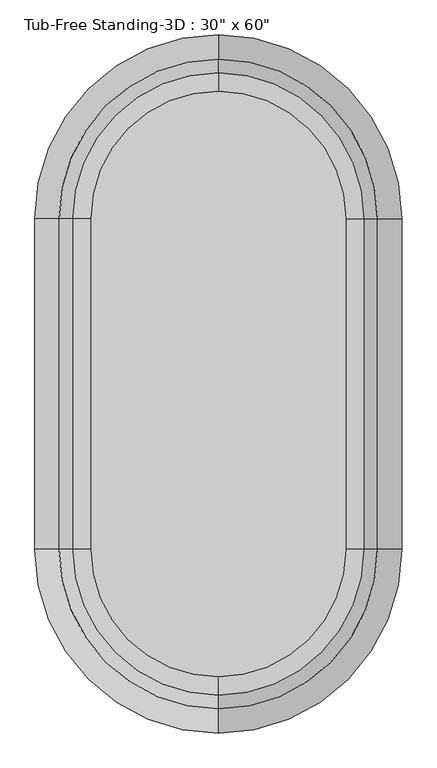
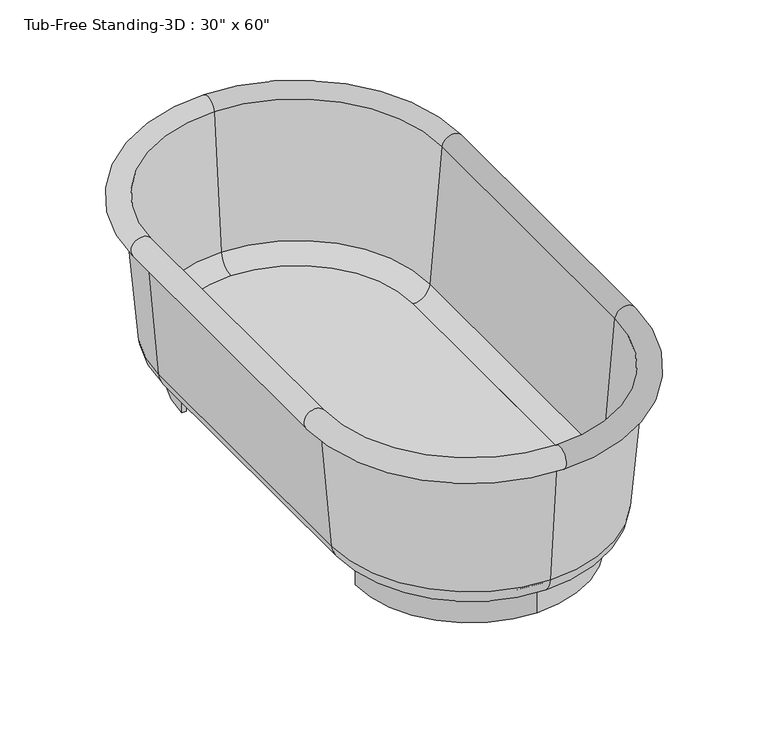
"""IFC4 building model written with IfcOpenShell, lengths in millimetres: flow terminal geometry."""

from ifc_helpers import new_model, si_unit, point, frame, frame_2d, origin, origin_with_axes, place, context, project, spatial, polyline, circle_curve, ellipse_curve, trimmed, segment, composite_curve, outline, extrude, source, transform, mapped, element, save
from ifc_brep_helpers import plane_surface, cylinder_surface, revolved_surface, advanced_brep


def flow_terminal_db991eef(model_context):
    return source(origin(), model_context, "Body", "SolidModel", [
        extrude(outline(composite_curve([segment(trimmed(circle_curve(frame_2d((0.0, 342.9)), 254.0), [point((0.0, 596.9))], [point((-254.0, 342.9))], True, "CARTESIAN"), True, "CONTINUOUS"), segment(polyline([(-254.0, 342.9), (-264.2824236, 342.9)]), True, "CONTINUOUS"), segment(trimmed(circle_curve(frame_2d((0.0, 342.9)), 264.2824236), [point((-264.2824236, 342.9))], [point((0.0, 607.1824236))], False, "CARTESIAN"), True, "CONTINUOUS"), segment(trimmed(circle_curve(frame_2d((0.0, 342.9)), 264.2824236), [point((0.0, 607.1824236))], [point((264.2824236, 342.9))], False, "CARTESIAN"), True, "CONTINUOUS"), segment(polyline([(264.2824236, 342.9), (254.0, 342.9)]), True, "CONTINUOUS"), segment(trimmed(circle_curve(frame_2d((0.0, 342.9)), 254.0), [point((254.0, 342.9))], [point((0.0, 596.9))], True, "CARTESIAN"), True, "CONTINUOUS")], self_intersect=False)), origin_with_axes(), (0.0, 0.0, 1.0), 63.5),
        extrude(outline(composite_curve([segment(trimmed(circle_curve(frame_2d((0.0, -342.9)), 264.2824236), [point((0.0, -607.1824236))], [point((-264.2824236, -342.9))], False, "CARTESIAN"), True, "CONTINUOUS"), segment(polyline([(-264.2824236, -342.9), (-254.0, -342.9)]), True, "CONTINUOUS"), segment(trimmed(circle_curve(frame_2d((0.0, -342.9)), 254.0), [point((-254.0, -342.9))], [point((0.0, -596.9))], True, "CARTESIAN"), True, "CONTINUOUS"), segment(trimmed(circle_curve(frame_2d((0.0, -342.9)), 254.0), [point((0.0, -596.9))], [point((254.0, -342.9))], True, "CARTESIAN"), True, "CONTINUOUS"), segment(polyline([(254.0, -342.9), (264.2824236, -342.9)]), True, "CONTINUOUS"), segment(trimmed(circle_curve(frame_2d((0.0, -342.9)), 264.2824236), [point((264.2824236, -342.9))], [point((0.0, -607.1824236))], False, "CARTESIAN"), True, "CONTINUOUS")], self_intersect=False)), origin_with_axes(), (0.0, 0.0, 1.0), 63.5),
        extrude(outline(composite_curve([segment(polyline([(-264.2824236, -342.9), (-264.2824236, 342.9)]), True, "CONTINUOUS"), segment(trimmed(circle_curve(frame_2d((0.0, 342.9)), 264.2824236), [point((-264.2824236, 342.9))], [point((0.0, 607.1824236))], False, "CARTESIAN"), True, "CONTINUOUS"), segment(trimmed(circle_curve(frame_2d((0.0, 342.9)), 264.2824236), [point((0.0, 607.1824236))], [point((264.2824236, 342.9))], False, "CARTESIAN"), True, "CONTINUOUS"), segment(polyline([(264.2824236, 342.9), (264.2824236, -342.9)]), True, "CONTINUOUS"), segment(trimmed(circle_curve(frame_2d((0.0, -342.9)), 264.2824236), [point((264.2824236, -342.9))], [point((0.0, -607.1824236))], False, "CARTESIAN"), True, "CONTINUOUS"), segment(trimmed(circle_curve(frame_2d((0.0, -342.9)), 264.2824236), [point((0.0, -607.1824236))], [point((-264.2824236, -342.9))], False, "CARTESIAN"), True, "CONTINUOUS")], self_intersect=False)), frame((0.0, 0.0, 63.5), z_axis=(0.0, 0.0, 1.0), x_axis=(1.0, 0.0, 0.0)), (0.0, 0.0, 1.0), 15.08125),
        advanced_brep(
        [(0.0, -685.8, 406.4), (342.9, -342.9, 406.4), (355.6, -342.9, 406.4), (0.0, -698.5, 406.4), (0.0, -660.0045038, 111.5561295), (317.1045038, -342.9, 111.5561295), (0.0, -607.1824236, 63.1536107), (264.2824236, -342.9, 63.1536107), (0.0, -607.1824236, 78.0774627), (264.2824236, -342.9, 78.0774627), (0.0, -645.1374416, 112.8568289), (302.2374416, -342.9, 112.8568289), (0.0, -673.3561556, 435.3982063), (330.4561556, -342.9, 435.3982063), (-342.9, -342.9, 406.4), (-355.6, -342.9, 406.4), (-317.1045038, -342.9, 111.5561295), (-264.2824236, -342.9, 63.1536107), (-264.2824236, -342.9, 78.0774627), (-302.2374416, -342.9, 112.8568289), (-330.4561556, -342.9, 435.3982063), (-355.6, 342.9, 406.4), (-342.9, 342.9, 406.4), (-317.1045038, 342.9, 111.5561295), (-264.2824236, 342.9, 63.1536107), (-264.2824236, 342.9, 78.0774627), (-302.2374416, 342.9, 112.8568289), (-330.4561556, 342.9, 435.3982063), (0.0, 685.8, 406.4), (0.0, 698.5, 406.4), (0.0, 660.0045038, 111.5561295), (0.0, 607.1824236, 63.1536107), (0.0, 607.1824236, 78.0774627), (0.0, 645.1374416, 112.8568289), (0.0, 673.3561556, 435.3982063), (342.9, 342.9, 406.4), (355.6, 342.9, 406.4), (317.1045038, 342.9, 111.5561295), (264.2824236, 342.9, 63.1536107), (264.2824236, 342.9, 78.0774627), (302.2374416, 342.9, 112.8568289), (330.4561556, 342.9, 435.3982063)],
        [
            (0, 1, circle_curve(frame((0.0, -342.9, 406.4), z_axis=(0.0, 0.0, 1.0), x_axis=(1.0, 0.0, 0.0)), 342.9)),
            (1, 2),
            (2, 3, circle_curve(frame((0.0, -342.9, 406.4), z_axis=(0.0, 0.0, -1.0), x_axis=(1.0, 0.0, 0.0)), 355.6)),
            (3, 0),
            (4, 5, circle_curve(frame((0.0, -342.9, 111.5561295), z_axis=(0.0, 0.0, 1.0), x_axis=(1.0, 0.0, 0.0)), 317.1045038)),
            (5, 1),
            (0, 4),
            (6, 7, circle_curve(frame((0.0, -342.9, 63.1536107), z_axis=(0.0, 0.0, 1.0), x_axis=(1.0, 0.0, 0.0)), 264.2824236)),
            (7, 5, circle_curve(frame((264.2824236, -342.9, 116.1774627), z_axis=(0.0, -1.0, 0.0), x_axis=(1.0, 0.0, 0.0)), 53.023852)),
            (4, 6, circle_curve(frame((0.0, -607.1824236, 116.1774627), z_axis=(1.0, 0.0, 0.0), x_axis=(0.0, -1.0, 0.0)), 53.023852)),
            (8, 9, circle_curve(frame((0.0, -342.9, 78.0774627), z_axis=(0.0, 0.0, 1.0), x_axis=(1.0, 0.0, 0.0)), 264.2824236)),
            (9, 7),
            (6, 8),
            (10, 11, circle_curve(frame((0.0, -342.9, 112.8568289), z_axis=(0.0, 0.0, 1.0), x_axis=(1.0, 0.0, 0.0)), 302.2374416)),
            (11, 9, circle_curve(frame((264.2824236, -342.9, 116.1774627), z_axis=(0.0, 1.0, 0.0), x_axis=(1.0, 0.0, 0.0)), 38.1)),
            (8, 10, circle_curve(frame((0.0, -607.1824236, 116.1774627), z_axis=(-1.0, 0.0, 0.0), x_axis=(0.0, -1.0, 0.0)), 38.1)),
            (12, 13, circle_curve(frame((0.0, -342.9, 435.3982063), z_axis=(0.0, 0.0, 1.0), x_axis=(1.0, 0.0, 0.0)), 330.4561556)),
            (13, 11),
            (10, 12),
            (2, 13, circle_curve(frame((355.6, -342.9, 431.8), z_axis=(0.0, -1.0, 0.0), x_axis=(1.0, 0.0, 0.0)), 25.4)),
            (12, 3, circle_curve(frame((0.0, -698.5, 431.8), z_axis=(1.0, 0.0, 0.0), x_axis=(0.0, -1.0, 0.0)), 25.4)),
            (14, 0, circle_curve(frame((0.0, -342.9, 406.4), z_axis=(0.0, 0.0, 1.0), x_axis=(0.0, -1.0, 0.0)), 342.9)),
            (3, 15, circle_curve(frame((0.0, -342.9, 406.4), z_axis=(0.0, 0.0, -1.0), x_axis=(0.0, -1.0, 0.0)), 355.6)),
            (15, 14),
            (16, 4, circle_curve(frame((0.0, -342.9, 111.5561295), z_axis=(0.0, 0.0, 1.0), x_axis=(0.0, -1.0, 0.0)), 317.1045038)),
            (14, 16),
            (17, 6, circle_curve(frame((0.0, -342.9, 63.1536107), z_axis=(0.0, 0.0, 1.0), x_axis=(0.0, -1.0, 0.0)), 264.2824236)),
            (16, 17, circle_curve(frame((-264.2824236, -342.9, 116.1774627), z_axis=(0.0, -1.0, 0.0), x_axis=(-1.0, 0.0, 0.0)), 53.023852)),
            (18, 8, circle_curve(frame((0.0, -342.9, 78.0774627), z_axis=(0.0, 0.0, 1.0), x_axis=(0.0, -1.0, 0.0)), 264.2824236)),
            (17, 18),
            (19, 10, circle_curve(frame((0.0, -342.9, 112.8568289), z_axis=(0.0, 0.0, 1.0), x_axis=(0.0, -1.0, 0.0)), 302.2374416)),
            (18, 19, circle_curve(frame((-264.2824236, -342.9, 116.1774627), z_axis=(0.0, 1.0, 0.0), x_axis=(-1.0, 0.0, 0.0)), 38.1)),
            (20, 12, circle_curve(frame((0.0, -342.9, 435.3982063), z_axis=(0.0, 0.0, 1.0), x_axis=(0.0, -1.0, 0.0)), 330.4561556)),
            (19, 20),
            (20, 15, circle_curve(frame((-355.6, -342.9, 431.8), z_axis=(0.0, -1.0, 0.0), x_axis=(-1.0, 0.0, 0.0)), 25.4)),
            (15, 21),
            (21, 22),
            (22, 14),
            (22, 23),
            (23, 16),
            (23, 24, circle_curve(frame((-264.2824236, 342.9, 116.1774627), z_axis=(0.0, -1.0, 0.0), x_axis=(-1.0, 0.0, 0.0)), 53.023852)),
            (24, 17),
            (24, 25),
            (25, 18),
            (25, 26, circle_curve(frame((-264.2824236, 342.9, 116.1774627), z_axis=(0.0, 1.0, 0.0), x_axis=(-1.0, 0.0, 0.0)), 38.1)),
            (26, 19),
            (26, 27),
            (27, 20),
            (27, 21, circle_curve(frame((-355.6, 342.9, 431.8), z_axis=(0.0, -1.0, 0.0), x_axis=(-1.0, 0.0, 0.0)), 25.4)),
            (28, 22, circle_curve(frame((0.0, 342.9, 406.4), z_axis=(0.0, 0.0, 1.0), x_axis=(-1.0, 0.0, 0.0)), 342.9)),
            (21, 29, circle_curve(frame((0.0, 342.9, 406.4), z_axis=(0.0, 0.0, -1.0), x_axis=(-1.0, 0.0, 0.0)), 355.6)),
            (29, 28),
            (30, 23, circle_curve(frame((0.0, 342.9, 111.5561295), z_axis=(0.0, 0.0, 1.0), x_axis=(-1.0, 0.0, 0.0)), 317.1045038)),
            (28, 30),
            (31, 24, circle_curve(frame((0.0, 342.9, 63.1536107), z_axis=(0.0, 0.0, 1.0), x_axis=(-1.0, 0.0, 0.0)), 264.2824236)),
            (30, 31, circle_curve(frame((0.0, 607.1824236, 116.1774627), z_axis=(-1.0, 0.0, 0.0), x_axis=(0.0, 1.0, 0.0)), 53.023852)),
            (32, 25, circle_curve(frame((0.0, 342.9, 78.0774627), z_axis=(0.0, 0.0, 1.0), x_axis=(-1.0, 0.0, 0.0)), 264.2824236)),
            (31, 32),
            (33, 26, circle_curve(frame((0.0, 342.9, 112.8568289), z_axis=(0.0, 0.0, 1.0), x_axis=(-1.0, 0.0, 0.0)), 302.2374416)),
            (32, 33, circle_curve(frame((0.0, 607.1824236, 116.1774627), z_axis=(1.0, 0.0, 0.0), x_axis=(0.0, 1.0, 0.0)), 38.1)),
            (34, 27, circle_curve(frame((0.0, 342.9, 435.3982063), z_axis=(0.0, 0.0, 1.0), x_axis=(-1.0, 0.0, 0.0)), 330.4561556)),
            (33, 34),
            (34, 29, circle_curve(frame((0.0, 698.5, 431.8), z_axis=(-1.0, 0.0, 0.0), x_axis=(0.0, 1.0, 0.0)), 25.4)),
            (35, 28, circle_curve(frame((0.0, 342.9, 406.4), z_axis=(0.0, 0.0, 1.0), x_axis=(0.0, 1.0, 0.0)), 342.9)),
            (29, 36, circle_curve(frame((0.0, 342.9, 406.4), z_axis=(0.0, 0.0, -1.0), x_axis=(0.0, 1.0, 0.0)), 355.6)),
            (36, 35),
            (37, 30, circle_curve(frame((0.0, 342.9, 111.5561295), z_axis=(0.0, 0.0, 1.0), x_axis=(0.0, 1.0, 0.0)), 317.1045038)),
            (35, 37),
            (38, 31, circle_curve(frame((0.0, 342.9, 63.1536107), z_axis=(0.0, 0.0, 1.0), x_axis=(0.0, 1.0, 0.0)), 264.2824236)),
            (37, 38, circle_curve(frame((264.2824236, 342.9, 116.1774627), z_axis=(0.0, 1.0, 0.0), x_axis=(1.0, 0.0, 0.0)), 53.023852)),
            (39, 32, circle_curve(frame((0.0, 342.9, 78.0774627), z_axis=(0.0, 0.0, 1.0), x_axis=(0.0, 1.0, 0.0)), 264.2824236)),
            (38, 39),
            (40, 33, circle_curve(frame((0.0, 342.9, 112.8568289), z_axis=(0.0, 0.0, 1.0), x_axis=(0.0, 1.0, 0.0)), 302.2374416)),
            (39, 40, circle_curve(frame((264.2824236, 342.9, 116.1774627), z_axis=(0.0, -1.0, 0.0), x_axis=(1.0, 0.0, 0.0)), 38.1)),
            (41, 34, circle_curve(frame((0.0, 342.9, 435.3982063), z_axis=(0.0, 0.0, 1.0), x_axis=(0.0, 1.0, 0.0)), 330.4561556)),
            (40, 41),
            (41, 36, circle_curve(frame((355.6, 342.9, 431.8), z_axis=(0.0, 1.0, 0.0), x_axis=(1.0, 0.0, 0.0)), 25.4)),
            (36, 2),
            (1, 35),
            (5, 37),
            (7, 38),
            (9, 39),
            (11, 40),
            (13, 41),
        ],
        [
            plane_surface(frame((0.0, -342.9, 406.4), z_axis=(0.0, 0.0, -1.0), x_axis=(1.0, 0.0, 0.0))),
            revolved_surface(polyline([(342.9, -342.9, 406.4), (317.1045038, -342.9, 111.5561295)]), (0.0, -342.9, 431.8), (0.0, 0.0, -1.0)),
            revolved_surface(trimmed(ellipse_curve(frame((264.2824236, -342.9, 116.1774627), z_axis=(0.0, 1.0, 0.0), x_axis=(1.0, 0.0, 0.0)), 53.023852, 53.023852), [point((317.1045038, -342.9, 111.5561295))], [point((264.2824236, -342.9, 63.1536107))], True, "CARTESIAN"), (0.0, -342.9, 431.8), (0.0, 0.0, -1.0)),
            revolved_surface(polyline([(264.2824236, -342.9, 63.1536107), (264.2824236, -342.9, 78.07746270000001)]), (0.0, -342.9, 431.8), (0.0, 0.0, -1.0)),
            revolved_surface(trimmed(ellipse_curve(frame((264.2824236, -342.9, 116.1774627), z_axis=(0.0, -1.0, 0.0), x_axis=(1.0, 0.0, 0.0)), 38.1, 38.1), [point((264.2824236, -342.9, 78.0774627))], [point((302.2374416, -342.9, 112.8568289))], True, "CARTESIAN"), (0.0, -342.9, 431.8), (0.0, 0.0, -1.0)),
            revolved_surface(polyline([(302.2374416, -342.9, 112.8568289), (330.4561556, -342.9, 435.3982063)]), (0.0, -342.9, 431.8), (0.0, 0.0, -1.0)),
            revolved_surface(trimmed(ellipse_curve(frame((355.6, -342.9, 431.8), z_axis=(0.0, 1.0, 0.0), x_axis=(1.0, 0.0, 0.0)), 25.4, 25.4), [point((330.4561556, -342.9, 435.3982063))], [point((355.6, -342.9, 406.4))], True, "CARTESIAN"), (0.0, -342.9, 431.8), (0.0, 0.0, -1.0)),
            plane_surface(frame((0.0, -342.9, 406.4), z_axis=(0.0, 0.0, -1.0), x_axis=(0.0, -1.0, 0.0))),
            revolved_surface(polyline([(0.0, -685.8, 406.4), (0.0, -660.0045038, 111.5561295)]), (0.0, -342.9, 431.8), (0.0, 0.0, -1.0)),
            revolved_surface(trimmed(ellipse_curve(frame((0.0, -607.1824236, 116.1774627), z_axis=(1.0, 0.0, 0.0), x_axis=(0.0, -1.0, 0.0)), 53.023852, 53.023852), [point((0.0, -660.0045038, 111.5561295))], [point((0.0, -607.1824236, 63.1536107))], True, "CARTESIAN"), (0.0, -342.9, 431.8), (0.0, 0.0, -1.0)),
            revolved_surface(polyline([(0.0, -607.1824236, 63.1536107), (0.0, -607.1824236, 78.07746270000001)]), (0.0, -342.9, 431.8), (0.0, 0.0, -1.0)),
            revolved_surface(trimmed(ellipse_curve(frame((0.0, -607.1824236, 116.1774627), z_axis=(-1.0, 0.0, 0.0), x_axis=(0.0, -1.0, 0.0)), 38.1, 38.1), [point((0.0, -607.1824236, 78.0774627))], [point((0.0, -645.1374416, 112.8568289))], True, "CARTESIAN"), (0.0, -342.9, 431.8), (0.0, 0.0, -1.0)),
            revolved_surface(polyline([(0.0, -645.1374416, 112.8568289), (0.0, -673.3561556, 435.3982063)]), (0.0, -342.9, 431.8), (0.0, 0.0, -1.0)),
            revolved_surface(trimmed(ellipse_curve(frame((0.0, -698.5, 431.8), z_axis=(1.0, 0.0, 0.0), x_axis=(0.0, -1.0, 0.0)), 25.4, 25.4), [point((0.0, -673.3561556, 435.3982063))], [point((0.0, -698.5, 406.4))], True, "CARTESIAN"), (0.0, -342.9, 431.8), (0.0, 0.0, -1.0)),
            plane_surface(frame((-355.6, -342.9, 406.4), z_axis=(0.0, 0.0, -1.0), x_axis=(0.0, 1.0, 0.0))),
            plane_surface(frame((-342.9, -342.9, 406.4), z_axis=(-0.9961946980917455, 0.0, -0.08715574274765871), x_axis=(0.0, 1.0, 0.0))),
            cylinder_surface(frame((-264.2824236, -342.9, 116.1774627), z_axis=(0.0, -1.0, 0.0), x_axis=(-1.0, 0.0, 0.0)), 53.023852),
            plane_surface(frame((-264.2824236, -342.9, 63.1536107), z_axis=(1.0, 0.0, 0.0), x_axis=(0.0, 1.0, 0.0))),
            revolved_surface(polyline([(-302.38242360000004, 342.9, 116.1774627), (-302.38242360000004, -342.9, 116.1774627)]), (-264.2824236, -342.9, 116.1774627), (0.0, 1.0, 0.0)),
            plane_surface(frame((-302.2374416, -342.9, 112.8568289), z_axis=(0.9961946980917458, 0.0, 0.08715574274765651), x_axis=(0.0, 1.0, 0.0))),
            cylinder_surface(frame((-355.6, -342.9, 431.8), z_axis=(0.0, -1.0, 0.0), x_axis=(-1.0, 0.0, 0.0)), 25.4),
            plane_surface(frame((0.0, 342.9, 406.4), z_axis=(0.0, 0.0, -1.0), x_axis=(-1.0, 0.0, 0.0))),
            revolved_surface(polyline([(-342.9, 342.9, 406.4), (-317.1045038, 342.9, 111.5561295)]), (0.0, 342.9, 431.8), (0.0, 0.0, -1.0)),
            revolved_surface(trimmed(ellipse_curve(frame((-264.2824236, 342.9, 116.1774627), z_axis=(0.0, -1.0, 0.0), x_axis=(-1.0, 0.0, 0.0)), 53.023852, 53.023852), [point((-317.1045038, 342.9, 111.5561295))], [point((-264.2824236, 342.9, 63.1536107))], True, "CARTESIAN"), (0.0, 342.9, 431.8), (0.0, 0.0, -1.0)),
            revolved_surface(polyline([(-264.2824236, 342.9, 63.1536107), (-264.2824236, 342.9, 78.07746270000001)]), (0.0, 342.9, 431.8), (0.0, 0.0, -1.0)),
            revolved_surface(trimmed(ellipse_curve(frame((-264.2824236, 342.9, 116.1774627), z_axis=(0.0, 1.0, 0.0), x_axis=(-1.0, 0.0, 0.0)), 38.1, 38.1), [point((-264.2824236, 342.9, 78.0774627))], [point((-302.2374416, 342.9, 112.8568289))], True, "CARTESIAN"), (0.0, 342.9, 431.8), (0.0, 0.0, -1.0)),
            revolved_surface(polyline([(-302.2374416, 342.9, 112.8568289), (-330.4561556, 342.9, 435.3982063)]), (0.0, 342.9, 431.8), (0.0, 0.0, -1.0)),
            revolved_surface(trimmed(ellipse_curve(frame((-355.6, 342.9, 431.8), z_axis=(0.0, -1.0, 0.0), x_axis=(-1.0, 0.0, 0.0)), 25.4, 25.4), [point((-330.4561556, 342.9, 435.3982063))], [point((-355.6, 342.9, 406.4))], True, "CARTESIAN"), (0.0, 342.9, 431.8), (0.0, 0.0, -1.0)),
            plane_surface(frame((0.0, 342.9, 406.4), z_axis=(0.0, 0.0, -1.0), x_axis=(0.0, 1.0, 0.0))),
            revolved_surface(polyline([(0.0, 685.8, 406.4), (0.0, 660.0045038, 111.5561295)]), (0.0, 342.9, 431.8), (0.0, 0.0, -1.0)),
            revolved_surface(trimmed(ellipse_curve(frame((0.0, 607.1824236, 116.1774627), z_axis=(-1.0, 0.0, 0.0), x_axis=(0.0, 1.0, 0.0)), 53.023852, 53.023852), [point((0.0, 660.0045038, 111.5561295))], [point((0.0, 607.1824236, 63.1536107))], True, "CARTESIAN"), (0.0, 342.9, 431.8), (0.0, 0.0, -1.0)),
            revolved_surface(polyline([(0.0, 607.1824236, 63.1536107), (0.0, 607.1824236, 78.07746270000001)]), (0.0, 342.9, 431.8), (0.0, 0.0, -1.0)),
            revolved_surface(trimmed(ellipse_curve(frame((0.0, 607.1824236, 116.1774627), z_axis=(1.0, 0.0, 0.0), x_axis=(0.0, 1.0, 0.0)), 38.1, 38.1), [point((0.0, 607.1824236, 78.0774627))], [point((0.0, 645.1374416, 112.8568289))], True, "CARTESIAN"), (0.0, 342.9, 431.8), (0.0, 0.0, -1.0)),
            revolved_surface(polyline([(0.0, 645.1374416, 112.8568289), (0.0, 673.3561556, 435.3982063)]), (0.0, 342.9, 431.8), (0.0, 0.0, -1.0)),
            revolved_surface(trimmed(ellipse_curve(frame((0.0, 698.5, 431.8), z_axis=(-1.0, 0.0, 0.0), x_axis=(0.0, 1.0, 0.0)), 25.4, 25.4), [point((0.0, 673.3561556, 435.3982063))], [point((0.0, 698.5, 406.4))], True, "CARTESIAN"), (0.0, 342.9, 431.8), (0.0, 0.0, -1.0)),
            plane_surface(frame((355.6, 342.9, 406.4), z_axis=(0.0, 0.0, -1.0), x_axis=(0.0, -1.0, 0.0))),
            plane_surface(frame((342.9, 342.9, 406.4), z_axis=(0.9961946980917455, 0.0, -0.08715574274765871), x_axis=(0.0, -1.0, 0.0))),
            cylinder_surface(frame((264.2824236, 342.9, 116.1774627), z_axis=(0.0, 1.0, 0.0), x_axis=(1.0, 0.0, 0.0)), 53.023852),
            plane_surface(frame((264.2824236, 342.9, 63.1536107), z_axis=(-1.0, 0.0, 0.0), x_axis=(0.0, -1.0, 0.0))),
            revolved_surface(polyline([(302.38242360000004, -342.9, 116.1774627), (302.38242360000004, 342.9, 116.1774627)]), (264.2824236, 342.9, 116.1774627), (0.0, -1.0, 0.0)),
            plane_surface(frame((302.2374416, 342.9, 112.8568289), z_axis=(-0.9961946980917458, 0.0, 0.08715574274765651), x_axis=(0.0, -1.0, 0.0))),
            cylinder_surface(frame((355.6, 342.9, 431.8), z_axis=(0.0, 1.0, 0.0), x_axis=(1.0, 0.0, 0.0)), 25.4),
        ],
        [
            (0, [[1, 2, 3, 4]]),
            (1, [[5, 6, -1, 7]]),
            (2, [[8, 9, -5, 10]]),
            (3, [[11, 12, -8, 13]]),
            (4, [[14, 15, -11, 16]]),
            (5, [[17, 18, -14, 19]]),
            (6, [[-3, 20, -17, 21]]),
            (7, [[22, -4, 23, 24]]),
            (8, [[25, -7, -22, 26]]),
            (9, [[27, -10, -25, 28]]),
            (10, [[29, -13, -27, 30]]),
            (11, [[31, -16, -29, 32]]),
            (12, [[33, -19, -31, 34]]),
            (13, [[-23, -21, -33, 35]]),
            (14, [[-24, 36, 37, 38]]),
            (15, [[-26, -38, 39, 40]]),
            (16, [[-28, -40, 41, 42]]),
            (17, [[-30, -42, 43, 44]]),
            (18, [[-32, -44, 45, 46]]),
            (19, [[-34, -46, 47, 48]]),
            (20, [[-35, -48, 49, -36]]),
            (21, [[50, -37, 51, 52]]),
            (22, [[53, -39, -50, 54]]),
            (23, [[55, -41, -53, 56]]),
            (24, [[57, -43, -55, 58]]),
            (25, [[59, -45, -57, 60]]),
            (26, [[61, -47, -59, 62]]),
            (27, [[-51, -49, -61, 63]]),
            (28, [[64, -52, 65, 66]]),
            (29, [[67, -54, -64, 68]]),
            (30, [[69, -56, -67, 70]]),
            (31, [[71, -58, -69, 72]]),
            (32, [[73, -60, -71, 74]]),
            (33, [[75, -62, -73, 76]]),
            (34, [[-65, -63, -75, 77]]),
            (35, [[-66, 78, -2, 79]]),
            (36, [[-68, -79, -6, 80]]),
            (37, [[-70, -80, -9, 81]]),
            (38, [[-72, -81, -12, 82]]),
            (39, [[-74, -82, -15, 83]]),
            (40, [[-76, -83, -18, 84]]),
            (41, [[-77, -84, -20, -78]]),
        ],
    ),
    ])


if __name__ == "__main__":
    model = new_model("IFC4")
    model_context = context("Model", 3, world=origin())
    ifc_project = project(units=[si_unit("LENGTHUNIT", "METRE", prefix="MILLI")], contexts=[model_context])
    site = spatial("IfcSite", under=ifc_project)
    building = spatial("IfcBuilding", under=site)
    placement = place(None, origin())
    flow_terminal_shape = flow_terminal_db991eef(model_context)
    element("IfcFlowTerminal", 1, ObjectType="Tub-Free Standing-3D : 30\" x 60\"", at=placement, inside=building, context=model_context, shape_type="MappedRepresentation", body=[
        mapped(flow_terminal_shape, transform((0.0, 0.0, 0.0), x_axis=(1.0, 0.0, 0.0), y_axis=(0.0, 1.0, 0.0), z_axis=(0.0, 0.0, 1.0))),
    ])
    save(model, "model.ifc")

# Revit data of these elements
# Type "Tub-Free Standing-3D : 30\" x 60\""
#   Assembly Code = "D2010110"
#   Height = 1' - 6"
#   Length = 4' - 9"
#   Width = 2' - 6"
#   Tub Material = Porcelain, Ivory
#   Default Elevation = 0
# Element 1 (IfcFlowTerminal, "Tub-Free Standing-3D : 30\" x 60\"")
#   Materials on its faces: "Porcelain, Ivory"
# Materials
#   "Porcelain, Ivory": class "Ceramic", colour RGB 247 247 239, transparency 0, Description = "Porcelain, ivory", Cost = 0
